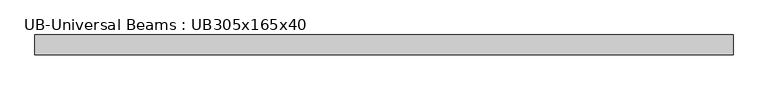
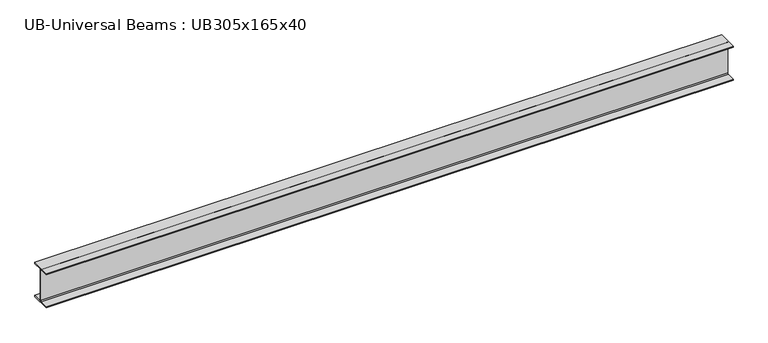
"""IFC4 building model written with IfcOpenShell, lengths in millimetres: beam geometry, UB-Universal Beams : UB305x165x40."""

from ifc_helpers import new_model, si_unit, point, frame, frame_2d, origin, place, context, project, spatial, polyline, circle_curve, trimmed, segment, composite_curve, outline, extrude, source, transform, mapped, element, save


def ub_universal_beams_ub305x165x40_3f70edd5(model_context):
    return source(origin(), model_context, "Body", "SweptSolid", [
        extrude(outline(composite_curve([segment(polyline([(82.5, -141.5), (82.5, -151.7), (-82.5, -151.7), (-82.5, -141.5), (-11.9, -141.5)]), True, "CONTINUOUS"), segment(trimmed(circle_curve(frame_2d((-11.9, -132.6)), 8.9), [point((-11.9, -141.5))], [point((-3.0, -132.6))], True, "CARTESIAN"), True, "CONTINUOUS"), segment(polyline([(-3.0, -132.6), (-3.0, 132.6)]), True, "CONTINUOUS"), segment(trimmed(circle_curve(frame_2d((-11.9, 132.6)), 8.9), [point((-3.0, 132.6))], [point((-11.9, 141.5))], True, "CARTESIAN"), True, "CONTINUOUS"), segment(polyline([(-11.9, 141.5), (-82.5, 141.5), (-82.5, 151.7), (82.5, 151.7), (82.5, 141.5), (11.9, 141.5)]), True, "CONTINUOUS"), segment(trimmed(circle_curve(frame_2d((11.9, 132.6)), 8.9), [point((11.9, 141.5))], [point((3.0, 132.6))], True, "CARTESIAN"), True, "CONTINUOUS"), segment(polyline([(3.0, 132.6), (3.0, -132.6)]), True, "CONTINUOUS"), segment(trimmed(circle_curve(frame_2d((11.9, -132.6)), 8.9), [point((3.0, -132.6))], [point((11.9, -141.5))], True, "CARTESIAN"), True, "CONTINUOUS"), segment(polyline([(11.9, -141.5), (82.5, -141.5)]), True, "CONTINUOUS")], self_intersect=False)), frame((-2881.3, 0.0, 0.0), z_axis=(1.0, 0.0, 0.0), x_axis=(0.0, 1.0, 0.0)), (0.0, 0.0, 1.0), 5762.6),
    ])


if __name__ == "__main__":
    model = new_model("IFC4")
    model_context = context("Model", 3, world=origin())
    ifc_project = project(units=[si_unit("LENGTHUNIT", "METRE", prefix="MILLI")], contexts=[model_context])
    site = spatial("IfcSite", under=ifc_project)
    building = spatial("IfcBuilding", under=site)
    placement = place(None, origin())
    ub_universal_beams_ub305x165x40_shape = ub_universal_beams_ub305x165x40_3f70edd5(model_context)
    element("IfcBeam", 1, ObjectType="UB-Universal Beams : UB305x165x40", at=placement, inside=building, context=model_context, shape_type="MappedRepresentation", body=[
        mapped(ub_universal_beams_ub305x165x40_shape, transform((0.0, 0.0, 0.0), x_axis=(1.0, 0.0, 0.0), y_axis=(0.0, 1.0, 0.0), z_axis=(0.0, 0.0, 1.0))),
    ])
    save(model, "model.ifc")

# Revit data of these elements
# Type "UB-Universal Beams : UB305x165x40"
#   Section Name Key = "UB305X165X40"
#   Width = 16.5 cm
#   Web Thickness = 0.6 cm
#   Web Fillet = 0.89 cm
#   Warping Constant = 164000.0 cm⁶
#   Torsional Moment of Inertia = 14.70 cm⁴
#   Section Area = 51.3 cm²
#   Plastic Modulus weak axis = 142.0 cm³
#   Plastic Modulus strong axis = 623.0 cm³
#   Nominal Weight = 40.2999 kgf/m
#   Moment of Inertia weak axis = 764.00 cm⁴
#   Moment of Inertia strong axis = 8503.00 cm⁴
#   Height = 30.34 cm
#   Flange Thickness = 1.02 cm
#   Elastic Modulus weak axis = 92.6 cm³
#   Elastic Modulus strong axis = 560.0 cm³
#   Centroid Vertical = 15.17 cm
#   Centroid Horizontal = 8.25 cm
#   Bolt Spacing = 9.0 cm
#   Length [instance default] = 1500 mm
#   Structural Material [instance default] = Metal - Steel 43-275
#   Type Comments = ""
#   Assembly Code = ""
# Element 1 (IfcBeam, "UB-Universal Beams : UB305x165x40")
#   Materials on its faces: "Metal - Steel 43-275"
# Materials
#   "Metal - Steel 43-275": class "Metal", colour RGB 247 247 247, transparency 0, Cost = 0
